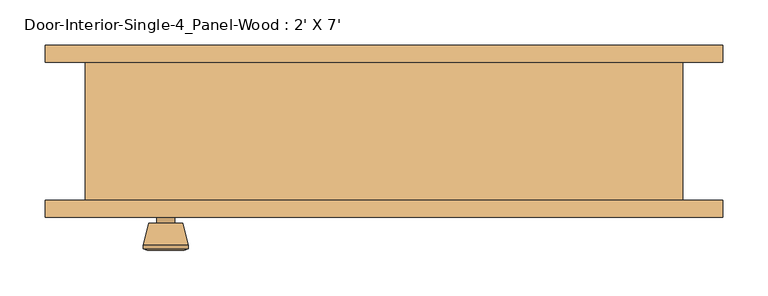
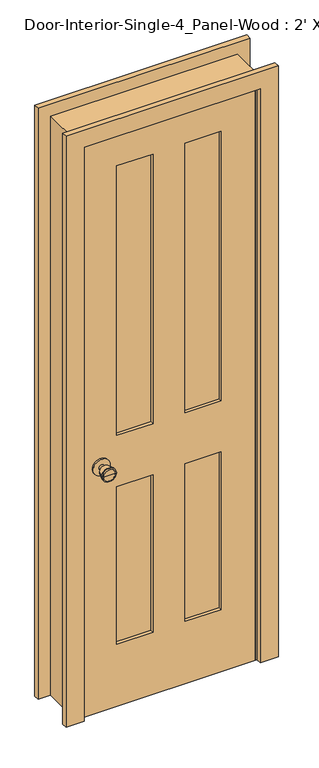
"""IFC4 building model written with IfcOpenShell, lengths in millimetres: door geometry, Door-Interior-Single-4_Panel-Wood : 2' X 7'."""

from ifc_helpers import new_model, si_unit, point, frame, frame_2d, origin, place, context, project, spatial, polyline, circle_curve, trimmed, segment, composite_curve, outline, extrude, faceted_brep, source, transform, mapped, element, save
from ifc_brep_helpers import plane_surface, cylinder_surface, revolved_surface, advanced_brep


def door_interior_single_4_panel_wood_2_x_7_0d1fc69e(model_context):
    return source(origin(), model_context, "Body", "SolidModel", [
        advanced_brep(
        [(-241.3, -32.1, 914.4), (-251.3, -32.1, 914.4), (-231.3, -32.1, 914.4), (-220.8241324, 16.9, 914.4), (-261.7758676, 16.9, 914.4), (-241.3, 16.9, 914.4), (-216.3, 15.0721319, 914.4), (-266.3, 15.0721319, 914.4), (-216.3, 11.6084537, 914.4), (-266.3, 11.6084537, 914.4), (-222.663764, -13.1, 914.4), (-259.936236, -13.1, 914.4), (-231.3, -13.1, 914.4), (-251.3, -13.1, 914.4)],
        [
            (0, 1),
            (1, 2, circle_curve(frame((-241.3, -32.1, 914.4), z_axis=(0.0, -1.0, 0.0), x_axis=(-1.0, 0.0, 0.0)), 10.0)),
            (2, 0),
            (2, 1, circle_curve(frame((-241.3, -32.1, 914.4), z_axis=(0.0, -1.0, 0.0), x_axis=(-1.0, 0.0, 0.0)), 10.0)),
            (3, 4, circle_curve(frame((-241.3, 16.9, 914.4), z_axis=(0.0, 1.0, 0.0), x_axis=(-1.0, 0.0, 0.0)), 20.4758676)),
            (4, 5),
            (5, 3),
            (4, 3, circle_curve(frame((-241.3, 16.9, 914.4), z_axis=(0.0, 1.0, 0.0), x_axis=(-1.0, 0.0, 0.0)), 20.4758676)),
            (6, 7, circle_curve(frame((-241.3, 15.0721319, 914.4), z_axis=(0.0, 1.0, 0.0), x_axis=(-1.0, 0.0, 0.0)), 25.0)),
            (7, 4),
            (3, 6),
            (7, 6, circle_curve(frame((-241.3, 15.0721319, 914.4), z_axis=(0.0, 1.0, 0.0), x_axis=(-1.0, 0.0, 0.0)), 25.0)),
            (8, 9, circle_curve(frame((-241.3, 11.6084537, 914.4), z_axis=(0.0, 1.0, 0.0), x_axis=(-1.0, 0.0, 0.0)), 25.0)),
            (9, 7),
            (6, 8),
            (9, 8, circle_curve(frame((-241.3, 11.6084537, 914.4), z_axis=(0.0, 1.0, 0.0), x_axis=(-1.0, 0.0, 0.0)), 25.0)),
            (10, 11, circle_curve(frame((-241.3, -13.1, 914.4), z_axis=(0.0, 1.0, 0.0), x_axis=(-1.0, 0.0, 0.0)), 18.636236)),
            (11, 9),
            (8, 10),
            (11, 10, circle_curve(frame((-241.3, -13.1, 914.4), z_axis=(0.0, 1.0, 0.0), x_axis=(-1.0, 0.0, 0.0)), 18.636236)),
            (12, 13, circle_curve(frame((-241.3, -13.1, 914.4), z_axis=(0.0, 1.0, 0.0), x_axis=(-1.0, 0.0, 0.0)), 10.0)),
            (13, 11),
            (10, 12),
            (13, 12, circle_curve(frame((-241.3, -13.1, 914.4), z_axis=(0.0, 1.0, 0.0), x_axis=(-1.0, 0.0, 0.0)), 10.0)),
            (1, 13),
            (12, 2),
        ],
        [
            plane_surface(frame((-241.3, -32.1, 914.4), z_axis=(0.0, -1.0, 0.0), x_axis=(-1.0, 0.0, 0.0))),
            plane_surface(frame((-241.3, 16.9, 914.4), z_axis=(0.0, 1.0, 0.0), x_axis=(-1.0, 0.0, 0.0))),
            revolved_surface(polyline([(-261.7758676, 16.9, 914.4), (-266.3, 15.0721319, 914.4)]), (-241.3, -32.1, 914.4), (0.0, -1.0, 0.0)),
            cylinder_surface(frame((-241.3, -32.1, 914.4), z_axis=(0.0, -1.0, 0.0), x_axis=(-1.0, 0.0, 0.0)), 25.0),
            revolved_surface(polyline([(-266.3, 11.6084537, 914.4), (-259.936236, -13.1, 914.4)]), (-241.3, -32.1, 914.4), (0.0, -1.0, 0.0)),
            plane_surface(frame((-241.3, -13.1, 914.4), z_axis=(0.0, -1.0, 0.0), x_axis=(-1.0, 0.0, 0.0))),
            cylinder_surface(frame((-241.3, -32.1, 914.4), z_axis=(0.0, -1.0, 0.0), x_axis=(-1.0, 0.0, 0.0)), 10.0),
        ],
        [
            (0, [[1, 2, 3]]),
            (0, [[-3, 4, -1]]),
            (1, [[5, 6, 7]]),
            (1, [[8, -7, -6]]),
            (2, [[9, 10, -5, 11]]),
            (2, [[12, -11, -8, -10]]),
            (3, [[13, 14, -9, 15]]),
            (3, [[16, -15, -12, -14]]),
            (4, [[17, 18, -13, 19]]),
            (4, [[20, -19, -16, -18]]),
            (5, [[21, 22, -17, 23]]),
            (5, [[24, -23, -20, -22]]),
            (6, [[-2, 25, -21, 26]]),
            (6, [[-4, -26, -24, -25]]),
        ],
    ),
        extrude(outline(composite_curve([segment(trimmed(circle_curve(frame_2d((914.4, -241.3)), 30.0), [point((914.4, -271.3))], [point((914.4, -211.3))], False, "CARTESIAN"), True, "CONTINUOUS"), segment(trimmed(circle_curve(frame_2d((914.4, -241.3)), 30.0), [point((914.4, -211.3))], [point((914.4, -271.3))], False, "CARTESIAN"), True, "CONTINUOUS")], self_intersect=False)), frame((0.0, -38.1, 0.0), z_axis=(0.0, 1.0, 0.0), x_axis=(0.0, 0.0, 1.0)), (0.0, 0.0, 1.0), 6.0),
        advanced_brep(
        [(-241.3, -79.025, 914.4), (-231.3, -79.025, 914.4), (-251.3, -79.025, 914.4), (-220.8241324, -128.025, 914.4), (-241.3, -128.025, 914.4), (-261.7758676, -128.025, 914.4), (-216.3, -126.1971319, 914.4), (-266.3, -126.1971319, 914.4), (-216.3, -122.7334537, 914.4), (-266.3, -122.7334537, 914.4), (-222.663764, -98.025, 914.4), (-259.936236, -98.025, 914.4), (-231.3, -98.025, 914.4), (-251.3, -98.025, 914.4)],
        [
            (0, 1),
            (1, 2, circle_curve(frame((-241.3, -79.025, 914.4), z_axis=(0.0, 1.0, 0.0), x_axis=(-1.0, 0.0, 0.0)), 10.0)),
            (2, 0),
            (2, 1, circle_curve(frame((-241.3, -79.025, 914.4), z_axis=(0.0, 1.0, 0.0), x_axis=(-1.0, 0.0, 0.0)), 10.0)),
            (3, 4),
            (4, 5),
            (5, 3, circle_curve(frame((-241.3, -128.025, 914.4), z_axis=(0.0, -1.0, 0.0), x_axis=(-1.0, 0.0, 0.0)), 20.4758676)),
            (3, 5, circle_curve(frame((-241.3, -128.025, 914.4), z_axis=(0.0, -1.0, 0.0), x_axis=(-1.0, 0.0, 0.0)), 20.4758676)),
            (6, 3),
            (5, 7),
            (7, 6, circle_curve(frame((-241.3, -126.1971319, 914.4), z_axis=(0.0, -1.0, 0.0), x_axis=(-1.0, 0.0, 0.0)), 25.0)),
            (6, 7, circle_curve(frame((-241.3, -126.1971319, 914.4), z_axis=(0.0, -1.0, 0.0), x_axis=(-1.0, 0.0, 0.0)), 25.0)),
            (8, 6),
            (7, 9),
            (9, 8, circle_curve(frame((-241.3, -122.7334537, 914.4), z_axis=(0.0, -1.0, 0.0), x_axis=(-1.0, 0.0, 0.0)), 25.0)),
            (8, 9, circle_curve(frame((-241.3, -122.7334537, 914.4), z_axis=(0.0, -1.0, 0.0), x_axis=(-1.0, 0.0, 0.0)), 25.0)),
            (10, 8),
            (9, 11),
            (11, 10, circle_curve(frame((-241.3, -98.025, 914.4), z_axis=(0.0, -1.0, 0.0), x_axis=(-1.0, 0.0, 0.0)), 18.636236)),
            (10, 11, circle_curve(frame((-241.3, -98.025, 914.4), z_axis=(0.0, -1.0, 0.0), x_axis=(-1.0, 0.0, 0.0)), 18.636236)),
            (12, 10),
            (11, 13),
            (13, 12, circle_curve(frame((-241.3, -98.025, 914.4), z_axis=(0.0, -1.0, 0.0), x_axis=(-1.0, 0.0, 0.0)), 10.0)),
            (12, 13, circle_curve(frame((-241.3, -98.025, 914.4), z_axis=(0.0, -1.0, 0.0), x_axis=(-1.0, 0.0, 0.0)), 10.0)),
            (1, 12),
            (13, 2),
        ],
        [
            plane_surface(frame((-241.3, -79.025, 914.4), z_axis=(0.0, 1.0, 0.0), x_axis=(-1.0, 0.0, 0.0))),
            plane_surface(frame((-241.3, -128.025, 914.4), z_axis=(0.0, -1.0, 0.0), x_axis=(-1.0, 0.0, 0.0))),
            revolved_surface(polyline([(-261.7758676, -128.025, 914.4), (-266.3, -126.1971319, 914.4)]), (-241.3, -79.025, 914.4), (0.0, 1.0, 0.0)),
            cylinder_surface(frame((-241.3, -79.025, 914.4), z_axis=(0.0, 1.0, 0.0), x_axis=(-1.0, 0.0, 0.0)), 25.0),
            revolved_surface(polyline([(-266.3, -122.7334537, 914.4), (-259.936236, -98.025, 914.4)]), (-241.3, -79.025, 914.4), (0.0, 1.0, 0.0)),
            plane_surface(frame((-241.3, -98.025, 914.4), z_axis=(0.0, 1.0, 0.0), x_axis=(-1.0, 0.0, 0.0))),
            cylinder_surface(frame((-241.3, -79.025, 914.4), z_axis=(0.0, 1.0, 0.0), x_axis=(-1.0, 0.0, 0.0)), 10.0),
        ],
        [
            (0, [[1, 2, 3]]),
            (0, [[-3, 4, -1]]),
            (1, [[5, 6, 7]]),
            (1, [[-6, -5, 8]]),
            (2, [[9, -7, 10, 11]]),
            (2, [[-10, -8, -9, 12]]),
            (3, [[13, -11, 14, 15]]),
            (3, [[-14, -12, -13, 16]]),
            (4, [[17, -15, 18, 19]]),
            (4, [[-18, -16, -17, 20]]),
            (5, [[21, -19, 22, 23]]),
            (5, [[-22, -20, -21, 24]]),
            (6, [[25, -23, 26, -2]]),
            (6, [[-26, -24, -25, -4]]),
        ],
    ),
        extrude(outline(composite_curve([segment(trimmed(circle_curve(frame_2d((914.4, -241.3)), 30.0), [point((914.4, -271.3))], [point((914.4, -211.3))], False, "CARTESIAN"), True, "CONTINUOUS"), segment(trimmed(circle_curve(frame_2d((914.4, -241.3)), 30.0), [point((914.4, -211.3))], [point((914.4, -271.3))], False, "CARTESIAN"), True, "CONTINUOUS")], self_intersect=False)), frame((0.0, -79.025, 0.0), z_axis=(0.0, 1.0, 0.0), x_axis=(0.0, 0.0, 1.0)), (0.0, 0.0, 1.0), 6.0),
        faceted_brep([(330.2, -73.025, 0.0), (304.8, -73.025, 0.0), (304.8, -38.1, 0.0), (292.1, -38.1, 0.0), (292.1, -3.175, 0.0), (304.8, -3.175, 0.0), (304.8, 79.375, 0.0), (330.2, 79.375, 0.0), (330.2, 79.375, 2159.0), (330.2, -73.025, 2159.0), (304.8, 79.375, 2133.6), (-304.8, 79.375, 2133.6), (-304.8, 79.375, 0.0), (-330.2, 79.375, 0.0), (-330.2, 79.375, 2159.0), (304.8, -3.175, 2133.6), (292.1, -3.175, 2120.9), (-292.1, -3.175, 2120.9), (-292.1, -3.175, 0.0), (-304.8, -3.175, 0.0), (-304.8, -3.175, 2133.6), (292.1, -38.1, 2120.9), (304.8, -38.1, 2133.6), (-304.8, -38.1, 2133.6), (-304.8, -38.1, 0.0), (-292.1, -38.1, 0.0), (-292.1, -38.1, 2120.9), (304.8, -73.025, 2133.6), (-330.2, -73.025, 2159.0), (-330.2, -73.025, 0.0), (-304.8, -73.025, 0.0), (-304.8, -73.025, 2133.6)], [[[0, 1, 2, 3, 4, 5, 6, 7]], [[7, 8, 9, 0]], [[6, 10, 11, 12, 13, 14, 8, 7]], [[5, 15, 10, 6]], [[4, 16, 17, 18, 19, 20, 15, 5]], [[3, 21, 16, 4]], [[2, 22, 23, 24, 25, 26, 21, 3]], [[1, 27, 22, 2]], [[0, 9, 28, 29, 30, 31, 27, 1]], [[8, 14, 28, 9]], [[15, 20, 11, 10]], [[21, 26, 17, 16]], [[27, 31, 23, 22]], [[29, 13, 12, 19, 18, 25, 24, 30]], [[14, 13, 29, 28]], [[20, 19, 12, 11]], [[26, 25, 18, 17]], [[31, 30, 24, 23]]]),
        extrude(outline(polyline([(2133.6, -304.8), (0.0, -304.8), (0.0, 304.8), (2133.6, 304.8), (2133.6, -304.8)]), holes=[polyline([(2014.5375, 57.15), (2014.5375, 184.15), (1009.65, 184.15), (1009.65, 57.15), (2014.5375, 57.15)]), polyline([(1009.65, -57.15), (1009.65, -184.15), (2014.5375, -184.15), (2014.5375, -57.15), (1009.65, -57.15)]), polyline([(819.15, 57.15), (819.15, 184.15), (231.775, 184.15), (231.775, 57.15), (819.15, 57.15)]), polyline([(231.775, -57.15), (231.775, -184.15), (819.15, -184.15), (819.15, -57.15), (231.775, -57.15)])]), frame((0.0, -73.025, 0.0), z_axis=(0.0, 1.0, 0.0), x_axis=(0.0, 0.0, 1.0)), (0.0, 0.0, 1.0), 34.925),
        extrude(outline(polyline([(184.15, -49.7416667), (184.15, -61.3833333), (57.15, -61.3833333), (57.15, -49.7416667), (184.15, -49.7416667)])), frame((0.0, 0.0, 1009.65), z_axis=(0.0, 0.0, 1.0), x_axis=(1.0, 0.0, 0.0)), (0.0, 0.0, 1.0), 1004.8875),
        extrude(outline(polyline([(-57.15, -49.7416667), (-57.15, -61.3833333), (-184.15, -61.3833333), (-184.15, -49.7416667), (-57.15, -49.7416667)])), frame((0.0, 0.0, 1009.65), z_axis=(0.0, 0.0, 1.0), x_axis=(1.0, 0.0, 0.0)), (0.0, 0.0, 1.0), 1004.8875),
        extrude(outline(polyline([(184.15, -49.7416667), (184.15, -61.3833333), (57.15, -61.3833333), (57.15, -49.7416667), (184.15, -49.7416667)])), frame((0.0, 0.0, 231.775), z_axis=(0.0, 0.0, 1.0), x_axis=(1.0, 0.0, 0.0)), (0.0, 0.0, 1.0), 587.375),
        extrude(outline(polyline([(-57.15, -49.7416667), (-57.15, -61.3833333), (-184.15, -61.3833333), (-184.15, -49.7416667), (-57.15, -49.7416667)])), frame((0.0, 0.0, 231.775), z_axis=(0.0, 0.0, 1.0), x_axis=(1.0, 0.0, 0.0)), (0.0, 0.0, 1.0), 587.375),
        extrude(outline(polyline([(0.0, 374.65), (2203.45, 374.65), (2203.45, -374.65), (0.0, -374.65), (0.0, -311.15), (2139.95, -311.15), (2139.95, 311.15), (0.0, 311.15), (0.0, 374.65)])), frame((0.0, -92.075, 0.0), z_axis=(0.0, 1.0, 0.0), x_axis=(0.0, 0.0, 1.0)), (0.0, 0.0, 1.0), 19.05),
        extrude(outline(polyline([(0.0, 374.65), (2203.45, 374.65), (2203.45, -374.65), (0.0, -374.65), (0.0, -311.15), (2139.95, -311.15), (2139.95, 311.15), (0.0, 311.15), (0.0, 374.65)])), frame((0.0, 79.375, 0.0), z_axis=(0.0, 1.0, 0.0), x_axis=(0.0, 0.0, 1.0)), (0.0, 0.0, 1.0), 19.05),
    ])


if __name__ == "__main__":
    model = new_model("IFC4")
    model_context = context("Model", 3, world=origin())
    ifc_project = project(units=[si_unit("LENGTHUNIT", "METRE", prefix="MILLI")], contexts=[model_context])
    site = spatial("IfcSite", under=ifc_project)
    building = spatial("IfcBuilding", under=site)
    placement = place(None, origin())
    door_interior_single_4_panel_wood_2_x_7_shape = door_interior_single_4_panel_wood_2_x_7_0d1fc69e(model_context)
    element("IfcDoor", 1, ObjectType="Door-Interior-Single-4_Panel-Wood : 2' X 7'", at=placement, inside=building, context=model_context, shape_type="MappedRepresentation", body=[
        mapped(door_interior_single_4_panel_wood_2_x_7_shape, transform((0.0, 0.0, 0.0), x_axis=(1.0, 0.0, 0.0), y_axis=(0.0, 1.0, 0.0), z_axis=(0.0, 0.0, 1.0))),
    ])
    save(model, "model.ifc")

# Revit data of these elements
# Type "Door-Interior-Single-4_Panel-Wood : 2' X 7'"
#   Type Mark = "17"
#   Assembly Code = "C1020300"
#   Analytic Construction = "Wooden"
#   Top Rail = 0' - 4 11/16"
#   Thickness = 0' - 1 3/8"
#   Thermal Resistance (R) = 2.5876 (h·ft²·°F)/BTU
#   Swing Angle [instance default] = 90.00°
#   Stiles = 0' - 4 3/4"
#   Rough Width = 2' - 2"
#   Rough Height = 7' - 1"
#   Mullion = 0' - 4 1/2"
#   Lock Rail = 0' - 7 1/2"
#   Height = 7' - 0"
#   Width = 2' - 0"
#   Heat Transfer Coefficient (U) = 0.3865 BTU/(h·ft²·°F)
#   Bottom Rail = 0' - 9 1/8"
#   Trim Material = Cherry
#   Panel Material = Cherry
#   Frame Material = Cherry
#   Door Handle Material = Aluminum
#   Visual Light Transmittance = 0
#   Solar Heat Gain Coefficient = 0
#   Wall Closure = (empty or 0)
#   Function = (empty or 0)
# Element 1 (IfcDoor, "Door-Interior-Single-4_Panel-Wood : 2' X 7'")
#   Materials on its faces: "Cherry", "Aluminum"
# Materials
#   "Cherry": class "Wood", colour RGB 226 177 128, transparency 0, Description = "Prunus Serotina", Cost = 0
#   "Aluminum": class "Metal", colour RGB 247 247 247, transparency 0, Description = "Aluminum 6061", Cost = 0
